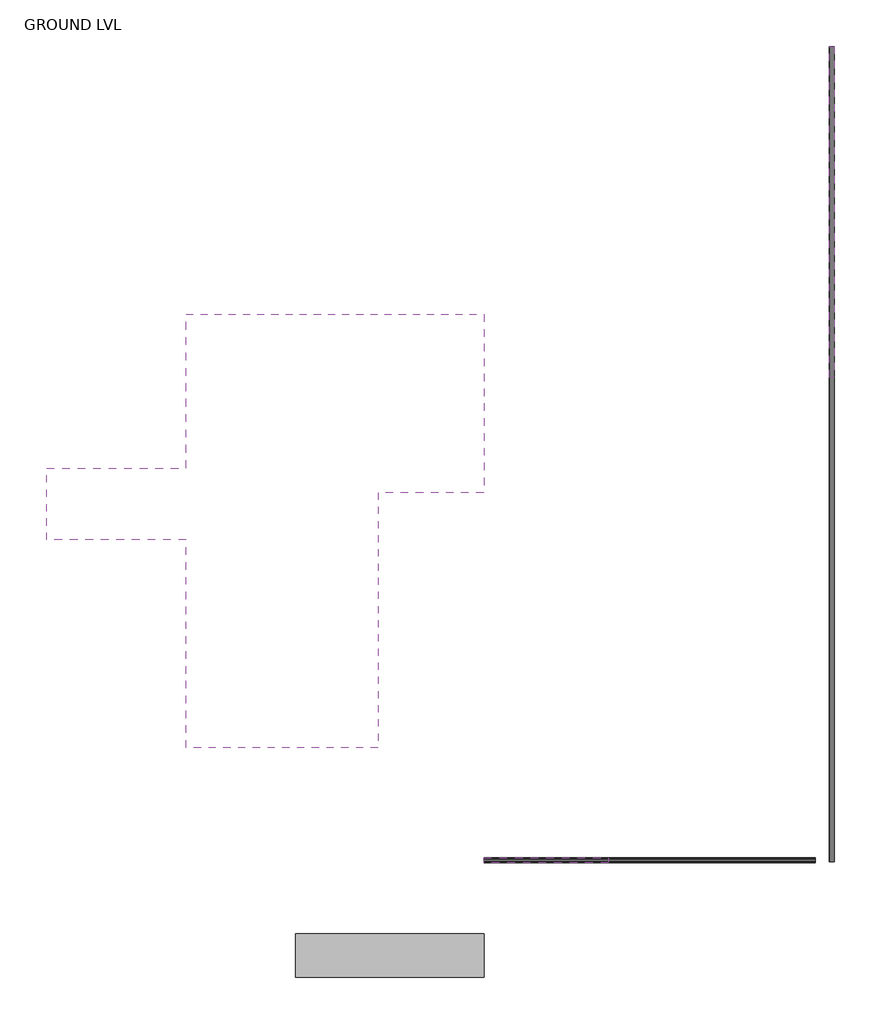
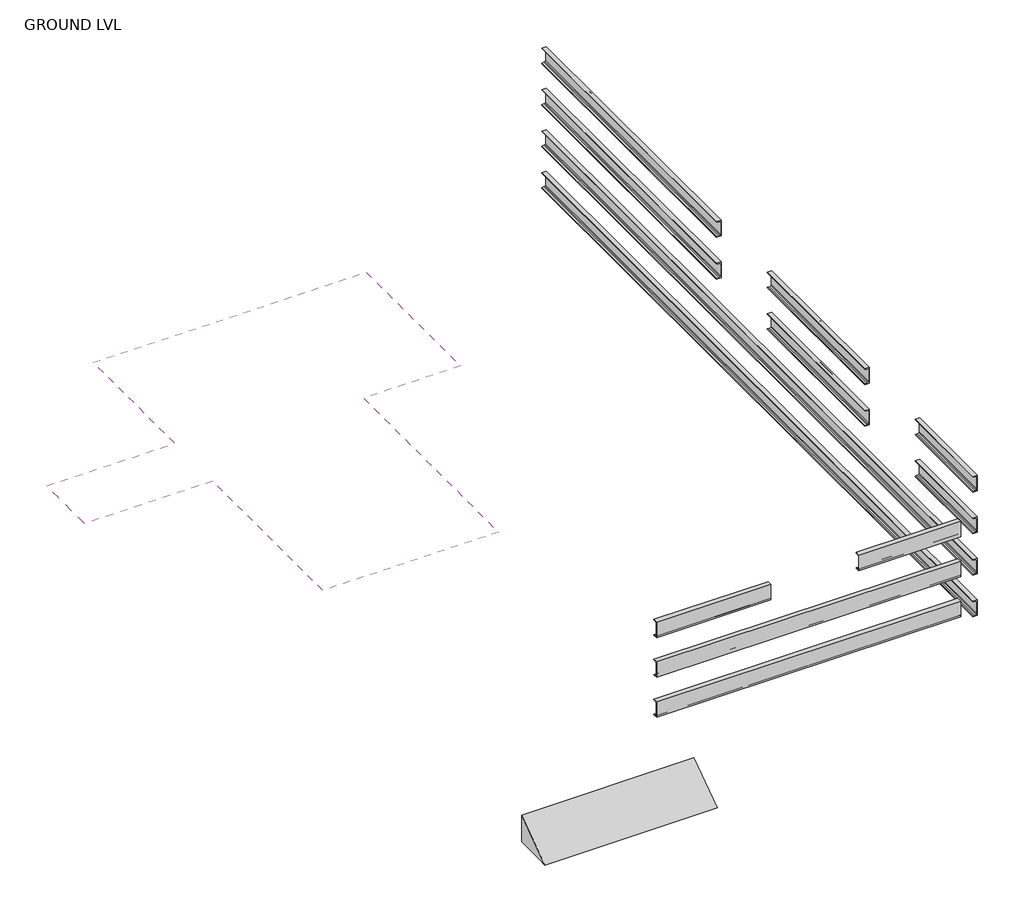
# One storey: 8 proxies, 1 covering.
"""IFC4 building model written with IfcOpenShell, lengths in millimetres."""

from ifc_helpers import new_model, si_unit, point, frame, frame_2d, origin, place, context, project, spatial, polyline, circle_curve, trimmed, segment, composite_curve, outline, extrude, transform, mapped, element, save
from components import generic_models_1_generic_models_1_f97e06e3

model = new_model("IFC4")

# Units and contexts
model_context = context("Model", 3, world=origin())
ifc_project = project(units=[si_unit("LENGTHUNIT", "METRE", prefix="MILLI")], contexts=[model_context])

# Site, building, storey
site = spatial("IfcSite", under=ifc_project)
building = spatial("IfcBuilding", under=site)
storey = spatial("IfcBuildingStorey", under=building, Name="GROUND LVL", Elevation=0.0)

# Proxies
placement = place(None, origin())
generic_models_1_generic_models_1_shape = generic_models_1_generic_models_1_f97e06e3(model_context)
element("IfcBuildingElementProxy", 1, Name="Generic Models 1 : Generic Models 1", ObjectType="Generic Models 1 : Generic Models 1", at=placement, inside=storey, context=model_context, shape_type="MappedRepresentation", body=[
    mapped(generic_models_1_generic_models_1_shape, transform((0.0, 0.0, 0.0), x_axis=(1.0, 0.0, 0.0), y_axis=(0.0, 1.0, 0.0), z_axis=(0.0, 0.0, 1.0))),
])
element("IfcBuildingElementProxy", 2, Name="Reveal", ObjectType="Reveal", at=placement, inside=storey, context=model_context, shape_type="SweptSolid", body=[
    extrude(outline(composite_curve([segment(polyline([(2425.7, -4738.2179867), (2425.7, -4801.4639867), (2424.3203242, -4801.4639867)]), True, "CONTINUOUS"), segment(trimmed(circle_curve(frame_2d((2424.3203242, -4796.2188867)), 5.2451), [point((2424.3203242, -4801.4639867))], [point((2419.1465897, -4797.0811775))], False, "CARTESIAN"), True, "CONTINUOUS"), segment(polyline([(2419.1465897, -4797.0811775), (2415.2098, -4773.4604867), (2412.00348, -4754.2226051)]), True, "CONTINUOUS"), segment(trimmed(circle_curve(frame_2d((2401.656011, -4755.9471867)), 10.4902), [point((2412.00348, -4754.2226051))], [point((2401.656011, -4745.4569867))], True, "CARTESIAN"), True, "CONTINUOUS"), segment(polyline([(2401.656011, -4745.4569867), (2221.143989, -4745.4569867)]), True, "CONTINUOUS"), segment(trimmed(circle_curve(frame_2d((2221.143989, -4755.9471867)), 10.4902), [point((2221.143989, -4745.4569867))], [point((2210.79652, -4754.2226051))], True, "CARTESIAN"), True, "CONTINUOUS"), segment(polyline([(2210.79652, -4754.2226051), (2207.5902, -4773.4604867), (2203.6534103, -4797.0811775)]), True, "CONTINUOUS"), segment(trimmed(circle_curve(frame_2d((2198.4796758, -4796.2188867)), 5.2451), [point((2203.6534103, -4797.0811775))], [point((2198.4796758, -4801.4639867))], False, "CARTESIAN"), True, "CONTINUOUS"), segment(polyline([(2198.4796758, -4801.4639867), (2197.1, -4801.4639867), (2197.1, -4738.2179867), (2425.7, -4738.2179867)]), True, "CONTINUOUS")], self_intersect=False)), frame((0.0, 4317.1500137, 0.0), z_axis=(0.0, 1.0, 0.0), x_axis=(0.0, 0.0, 1.0)), (0.0, 0.0, 1.0), 4203.7),
    extrude(outline(composite_curve([segment(polyline([(2425.7, -4738.2179867), (2425.7, -4801.4639867), (2424.3203242, -4801.4639867)]), True, "CONTINUOUS"), segment(trimmed(circle_curve(frame_2d((2424.3203242, -4796.2188867)), 5.2451), [point((2424.3203242, -4801.4639867))], [point((2419.1465897, -4797.0811775))], False, "CARTESIAN"), True, "CONTINUOUS"), segment(polyline([(2419.1465897, -4797.0811775), (2415.2098, -4773.4604867), (2412.00348, -4754.2226051)]), True, "CONTINUOUS"), segment(trimmed(circle_curve(frame_2d((2401.656011, -4755.9471867)), 10.4902), [point((2412.00348, -4754.2226051))], [point((2401.656011, -4745.4569867))], True, "CARTESIAN"), True, "CONTINUOUS"), segment(polyline([(2401.656011, -4745.4569867), (2221.143989, -4745.4569867)]), True, "CONTINUOUS"), segment(trimmed(circle_curve(frame_2d((2221.143989, -4755.9471867)), 10.4902), [point((2221.143989, -4745.4569867))], [point((2210.79652, -4754.2226051))], True, "CARTESIAN"), True, "CONTINUOUS"), segment(polyline([(2210.79652, -4754.2226051), (2207.5902, -4773.4604867), (2203.6534103, -4797.0811775)]), True, "CONTINUOUS"), segment(trimmed(circle_curve(frame_2d((2198.4796758, -4796.2188867)), 5.2451), [point((2203.6534103, -4797.0811775))], [point((2198.4796758, -4801.4639867))], False, "CARTESIAN"), True, "CONTINUOUS"), segment(polyline([(2198.4796758, -4801.4639867), (2197.1, -4801.4639867), (2197.1, -4738.2179867), (2425.7, -4738.2179867)]), True, "CONTINUOUS")], self_intersect=False)), frame((0.0, 761.1500137, 0.0), z_axis=(0.0, 1.0, 0.0), x_axis=(0.0, 0.0, 1.0)), (0.0, 0.0, 1.0), 2336.8),
    extrude(outline(composite_curve([segment(polyline([(2425.7, -4738.2179867), (2425.7, -4801.4639867), (2424.3203242, -4801.4639867)]), True, "CONTINUOUS"), segment(trimmed(circle_curve(frame_2d((2424.3203242, -4796.2188867)), 5.2451), [point((2424.3203242, -4801.4639867))], [point((2419.1465897, -4797.0811775))], False, "CARTESIAN"), True, "CONTINUOUS"), segment(polyline([(2419.1465897, -4797.0811775), (2415.2098, -4773.4604867), (2412.00348, -4754.2226051)]), True, "CONTINUOUS"), segment(trimmed(circle_curve(frame_2d((2401.656011, -4755.9471867)), 10.4902), [point((2412.00348, -4754.2226051))], [point((2401.656011, -4745.4569867))], True, "CARTESIAN"), True, "CONTINUOUS"), segment(polyline([(2401.656011, -4745.4569867), (2221.143989, -4745.4569867)]), True, "CONTINUOUS"), segment(trimmed(circle_curve(frame_2d((2221.143989, -4755.9471867)), 10.4902), [point((2221.143989, -4745.4569867))], [point((2210.79652, -4754.2226051))], True, "CARTESIAN"), True, "CONTINUOUS"), segment(polyline([(2210.79652, -4754.2226051), (2207.5902, -4773.4604867), (2203.6534103, -4797.0811775)]), True, "CONTINUOUS"), segment(trimmed(circle_curve(frame_2d((2198.4796758, -4796.2188867)), 5.2451), [point((2203.6534103, -4797.0811775))], [point((2198.4796758, -4801.4639867))], False, "CARTESIAN"), True, "CONTINUOUS"), segment(polyline([(2198.4796758, -4801.4639867), (2197.1, -4801.4639867), (2197.1, -4738.2179867), (2425.7, -4738.2179867)]), True, "CONTINUOUS")], self_intersect=False)), frame((0.0, -1842.3499863, 0.0), z_axis=(0.0, 1.0, 0.0), x_axis=(0.0, 0.0, 1.0)), (0.0, 0.0, 1.0), 1384.3),
])
element("IfcBuildingElementProxy", 3, Name="Reveal", ObjectType="Reveal", at=placement, inside=storey, context=model_context, shape_type="SweptSolid", body=[
    extrude(outline(composite_curve([segment(polyline([(-1857.2343863, 1841.5), (-1793.9883863, 1841.5), (-1793.9883863, 1840.1203242)]), True, "CONTINUOUS"), segment(trimmed(circle_curve(frame_2d((-1799.2334863, 1840.1203242)), 5.2451), [point((-1793.9883863, 1840.1203242))], [point((-1798.3711955, 1834.9465897))], False, "CARTESIAN"), True, "CONTINUOUS"), segment(polyline([(-1798.3711955, 1834.9465897), (-1821.9918863, 1831.0098), (-1841.2297679, 1827.80348)]), True, "CONTINUOUS"), segment(trimmed(circle_curve(frame_2d((-1839.5051863, 1817.456011)), 10.4902), [point((-1841.2297679, 1827.80348))], [point((-1849.9953863, 1817.456011))], True, "CARTESIAN"), True, "CONTINUOUS"), segment(polyline([(-1849.9953863, 1817.456011), (-1849.9953863, 1636.943989)]), True, "CONTINUOUS"), segment(trimmed(circle_curve(frame_2d((-1839.5051863, 1636.943989)), 10.4902), [point((-1849.9953863, 1636.943989))], [point((-1841.2297679, 1626.59652))], True, "CARTESIAN"), True, "CONTINUOUS"), segment(polyline([(-1841.2297679, 1626.59652), (-1821.9918863, 1623.3902), (-1798.3711955, 1619.4534103)]), True, "CONTINUOUS"), segment(trimmed(circle_curve(frame_2d((-1799.2334863, 1614.2796758)), 5.2451), [point((-1798.3711955, 1619.4534103))], [point((-1793.9883863, 1614.2796758))], False, "CARTESIAN"), True, "CONTINUOUS"), segment(polyline([(-1793.9883863, 1614.2796758), (-1793.9883863, 1612.9), (-1857.2343863, 1612.9), (-1857.2343863, 1841.5)]), True, "CONTINUOUS")], self_intersect=False)), frame((-6391.4023867, 0.0, 0.0), z_axis=(1.0, 0.0, 0.0), x_axis=(0.0, 1.0, 0.0)), (0.0, 0.0, 1.0), 1409.7),
    extrude(outline(composite_curve([segment(polyline([(-1857.2343863, 1841.5), (-1793.9883863, 1841.5), (-1793.9883863, 1840.1203242)]), True, "CONTINUOUS"), segment(trimmed(circle_curve(frame_2d((-1799.2334863, 1840.1203242)), 5.2451), [point((-1793.9883863, 1840.1203242))], [point((-1798.3711955, 1834.9465897))], False, "CARTESIAN"), True, "CONTINUOUS"), segment(polyline([(-1798.3711955, 1834.9465897), (-1821.9918863, 1831.0098), (-1841.2297679, 1827.80348)]), True, "CONTINUOUS"), segment(trimmed(circle_curve(frame_2d((-1839.5051863, 1817.456011)), 10.4902), [point((-1841.2297679, 1827.80348))], [point((-1849.9953863, 1817.456011))], True, "CARTESIAN"), True, "CONTINUOUS"), segment(polyline([(-1849.9953863, 1817.456011), (-1849.9953863, 1636.943989)]), True, "CONTINUOUS"), segment(trimmed(circle_curve(frame_2d((-1839.5051863, 1636.943989)), 10.4902), [point((-1849.9953863, 1636.943989))], [point((-1841.2297679, 1626.59652))], True, "CARTESIAN"), True, "CONTINUOUS"), segment(polyline([(-1841.2297679, 1626.59652), (-1821.9918863, 1623.3902), (-1798.3711955, 1619.4534103)]), True, "CONTINUOUS"), segment(trimmed(circle_curve(frame_2d((-1799.2334863, 1614.2796758)), 5.2451), [point((-1798.3711955, 1619.4534103))], [point((-1793.9883863, 1614.2796758))], False, "CARTESIAN"), True, "CONTINUOUS"), segment(polyline([(-1793.9883863, 1614.2796758), (-1793.9883863, 1612.9), (-1857.2343863, 1612.9), (-1857.2343863, 1841.5)]), True, "CONTINUOUS")], self_intersect=False)), frame((-9198.1023867, 0.0, 0.0), z_axis=(1.0, 0.0, 0.0), x_axis=(0.0, 1.0, 0.0)), (0.0, 0.0, 1.0), 1587.5),
])
element("IfcBuildingElementProxy", 4, Name="Reveal", ObjectType="Reveal", at=placement, inside=storey, context=model_context, shape_type="SweptSolid", body=[
    extrude(outline(composite_curve([segment(polyline([(-1857.2343863, 1257.3), (-1793.9883863, 1257.3), (-1793.9883863, 1255.9203242)]), True, "CONTINUOUS"), segment(trimmed(circle_curve(frame_2d((-1799.2334863, 1255.9203242)), 5.2451), [point((-1793.9883863, 1255.9203242))], [point((-1798.3711955, 1250.7465897))], False, "CARTESIAN"), True, "CONTINUOUS"), segment(polyline([(-1798.3711955, 1250.7465897), (-1821.9918863, 1246.8098), (-1841.2297679, 1243.60348)]), True, "CONTINUOUS"), segment(trimmed(circle_curve(frame_2d((-1839.5051863, 1233.256011)), 10.4902), [point((-1841.2297679, 1243.60348))], [point((-1849.9953863, 1233.256011))], True, "CARTESIAN"), True, "CONTINUOUS"), segment(polyline([(-1849.9953863, 1233.256011), (-1849.9953863, 1052.743989)]), True, "CONTINUOUS"), segment(trimmed(circle_curve(frame_2d((-1839.5051863, 1052.743989)), 10.4902), [point((-1849.9953863, 1052.743989))], [point((-1841.2297679, 1042.39652))], True, "CARTESIAN"), True, "CONTINUOUS"), segment(polyline([(-1841.2297679, 1042.39652), (-1821.9918863, 1039.1902), (-1798.3711955, 1035.2534103)]), True, "CONTINUOUS"), segment(trimmed(circle_curve(frame_2d((-1799.2334863, 1030.0796758)), 5.2451), [point((-1798.3711955, 1035.2534103))], [point((-1793.9883863, 1030.0796758))], False, "CARTESIAN"), True, "CONTINUOUS"), segment(polyline([(-1793.9883863, 1030.0796758), (-1793.9883863, 1028.7), (-1857.2343863, 1028.7), (-1857.2343863, 1257.3)]), True, "CONTINUOUS")], self_intersect=False)), frame((-9198.1023867, 0.0, 0.0), z_axis=(1.0, 0.0, 0.0), x_axis=(0.0, 1.0, 0.0)), (0.0, 0.0, 1.0), 4216.4),
])
element("IfcBuildingElementProxy", 5, Name="Reveal", ObjectType="Reveal", at=placement, inside=storey, context=model_context, shape_type="SweptSolid", body=[
    extrude(outline(composite_curve([segment(polyline([(-1857.2343863, 673.1), (-1793.9883863, 673.1), (-1793.9883863, 671.7203242)]), True, "CONTINUOUS"), segment(trimmed(circle_curve(frame_2d((-1799.2334863, 671.7203242)), 5.2451), [point((-1793.9883863, 671.7203242))], [point((-1798.3711955, 666.5465897))], False, "CARTESIAN"), True, "CONTINUOUS"), segment(polyline([(-1798.3711955, 666.5465897), (-1821.9918863, 662.6098), (-1841.2297679, 659.40348)]), True, "CONTINUOUS"), segment(trimmed(circle_curve(frame_2d((-1839.5051863, 649.056011)), 10.4902), [point((-1841.2297679, 659.40348))], [point((-1849.9953863, 649.056011))], True, "CARTESIAN"), True, "CONTINUOUS"), segment(polyline([(-1849.9953863, 649.056011), (-1849.9953863, 468.543989)]), True, "CONTINUOUS"), segment(trimmed(circle_curve(frame_2d((-1839.5051863, 468.543989)), 10.4902), [point((-1849.9953863, 468.543989))], [point((-1841.2297679, 458.19652))], True, "CARTESIAN"), True, "CONTINUOUS"), segment(polyline([(-1841.2297679, 458.19652), (-1821.9918863, 454.9902), (-1798.3711955, 451.0534103)]), True, "CONTINUOUS"), segment(trimmed(circle_curve(frame_2d((-1799.2334863, 445.8796758)), 5.2451), [point((-1798.3711955, 451.0534103))], [point((-1793.9883863, 445.8796758))], False, "CARTESIAN"), True, "CONTINUOUS"), segment(polyline([(-1793.9883863, 445.8796758), (-1793.9883863, 444.5), (-1857.2343863, 444.5), (-1857.2343863, 673.1)]), True, "CONTINUOUS")], self_intersect=False)), frame((-9198.1023867, 0.0, 0.0), z_axis=(1.0, 0.0, 0.0), x_axis=(0.0, 1.0, 0.0)), (0.0, 0.0, 1.0), 4216.4),
])
element("IfcBuildingElementProxy", 6, Name="Reveal", ObjectType="Reveal", at=placement, inside=storey, context=model_context, shape_type="SweptSolid", body=[
    extrude(outline(composite_curve([segment(polyline([(1816.1, -4738.2179867), (1816.1, -4801.4639867), (1814.7203242, -4801.4639867)]), True, "CONTINUOUS"), segment(trimmed(circle_curve(frame_2d((1814.7203242, -4796.2188867)), 5.2451), [point((1814.7203242, -4801.4639867))], [point((1809.5465897, -4797.0811775))], False, "CARTESIAN"), True, "CONTINUOUS"), segment(polyline([(1809.5465897, -4797.0811775), (1805.6098, -4773.4604867), (1802.40348, -4754.2226051)]), True, "CONTINUOUS"), segment(trimmed(circle_curve(frame_2d((1792.056011, -4755.9471867)), 10.4902), [point((1802.40348, -4754.2226051))], [point((1792.056011, -4745.4569867))], True, "CARTESIAN"), True, "CONTINUOUS"), segment(polyline([(1792.056011, -4745.4569867), (1611.543989, -4745.4569867)]), True, "CONTINUOUS"), segment(trimmed(circle_curve(frame_2d((1611.543989, -4755.9471867)), 10.4902), [point((1611.543989, -4745.4569867))], [point((1601.19652, -4754.2226051))], True, "CARTESIAN"), True, "CONTINUOUS"), segment(polyline([(1601.19652, -4754.2226051), (1597.9902, -4773.4604867), (1594.0534103, -4797.0811775)]), True, "CONTINUOUS"), segment(trimmed(circle_curve(frame_2d((1588.8796758, -4796.2188867)), 5.2451), [point((1594.0534103, -4797.0811775))], [point((1588.8796758, -4801.4639867))], False, "CARTESIAN"), True, "CONTINUOUS"), segment(polyline([(1588.8796758, -4801.4639867), (1587.5, -4801.4639867), (1587.5, -4738.2179867), (1816.1, -4738.2179867)]), True, "CONTINUOUS")], self_intersect=False)), frame((0.0, 4317.1500137, 0.0), z_axis=(0.0, 1.0, 0.0), x_axis=(0.0, 0.0, 1.0)), (0.0, 0.0, 1.0), 4203.7),
    extrude(outline(composite_curve([segment(polyline([(1816.1, -4738.2179867), (1816.1, -4801.4639867), (1814.7203242, -4801.4639867)]), True, "CONTINUOUS"), segment(trimmed(circle_curve(frame_2d((1814.7203242, -4796.2188867)), 5.2451), [point((1814.7203242, -4801.4639867))], [point((1809.5465897, -4797.0811775))], False, "CARTESIAN"), True, "CONTINUOUS"), segment(polyline([(1809.5465897, -4797.0811775), (1805.6098, -4773.4604867), (1802.40348, -4754.2226051)]), True, "CONTINUOUS"), segment(trimmed(circle_curve(frame_2d((1792.056011, -4755.9471867)), 10.4902), [point((1802.40348, -4754.2226051))], [point((1792.056011, -4745.4569867))], True, "CARTESIAN"), True, "CONTINUOUS"), segment(polyline([(1792.056011, -4745.4569867), (1611.543989, -4745.4569867)]), True, "CONTINUOUS"), segment(trimmed(circle_curve(frame_2d((1611.543989, -4755.9471867)), 10.4902), [point((1611.543989, -4745.4569867))], [point((1601.19652, -4754.2226051))], True, "CARTESIAN"), True, "CONTINUOUS"), segment(polyline([(1601.19652, -4754.2226051), (1597.9902, -4773.4604867), (1594.0534103, -4797.0811775)]), True, "CONTINUOUS"), segment(trimmed(circle_curve(frame_2d((1588.8796758, -4796.2188867)), 5.2451), [point((1594.0534103, -4797.0811775))], [point((1588.8796758, -4801.4639867))], False, "CARTESIAN"), True, "CONTINUOUS"), segment(polyline([(1588.8796758, -4801.4639867), (1587.5, -4801.4639867), (1587.5, -4738.2179867), (1816.1, -4738.2179867)]), True, "CONTINUOUS")], self_intersect=False)), frame((0.0, 761.1500137, 0.0), z_axis=(0.0, 1.0, 0.0), x_axis=(0.0, 0.0, 1.0)), (0.0, 0.0, 1.0), 2336.8),
    extrude(outline(composite_curve([segment(polyline([(1816.1, -4738.2179867), (1816.1, -4801.4639867), (1814.7203242, -4801.4639867)]), True, "CONTINUOUS"), segment(trimmed(circle_curve(frame_2d((1814.7203242, -4796.2188867)), 5.2451), [point((1814.7203242, -4801.4639867))], [point((1809.5465897, -4797.0811775))], False, "CARTESIAN"), True, "CONTINUOUS"), segment(polyline([(1809.5465897, -4797.0811775), (1805.6098, -4773.4604867), (1802.40348, -4754.2226051)]), True, "CONTINUOUS"), segment(trimmed(circle_curve(frame_2d((1792.056011, -4755.9471867)), 10.4902), [point((1802.40348, -4754.2226051))], [point((1792.056011, -4745.4569867))], True, "CARTESIAN"), True, "CONTINUOUS"), segment(polyline([(1792.056011, -4745.4569867), (1611.543989, -4745.4569867)]), True, "CONTINUOUS"), segment(trimmed(circle_curve(frame_2d((1611.543989, -4755.9471867)), 10.4902), [point((1611.543989, -4745.4569867))], [point((1601.19652, -4754.2226051))], True, "CARTESIAN"), True, "CONTINUOUS"), segment(polyline([(1601.19652, -4754.2226051), (1597.9902, -4773.4604867), (1594.0534103, -4797.0811775)]), True, "CONTINUOUS"), segment(trimmed(circle_curve(frame_2d((1588.8796758, -4796.2188867)), 5.2451), [point((1594.0534103, -4797.0811775))], [point((1588.8796758, -4801.4639867))], False, "CARTESIAN"), True, "CONTINUOUS"), segment(polyline([(1588.8796758, -4801.4639867), (1587.5, -4801.4639867), (1587.5, -4738.2179867), (1816.1, -4738.2179867)]), True, "CONTINUOUS")], self_intersect=False)), frame((0.0, -1842.3499863, 0.0), z_axis=(0.0, 1.0, 0.0), x_axis=(0.0, 0.0, 1.0)), (0.0, 0.0, 1.0), 1384.3),
])
element("IfcBuildingElementProxy", 7, Name="Reveal", ObjectType="Reveal", at=placement, inside=storey, context=model_context, shape_type="SweptSolid", body=[
    extrude(outline(composite_curve([segment(polyline([(1206.5, -4738.2179867), (1206.5, -4801.4639867), (1205.1203242, -4801.4639867)]), True, "CONTINUOUS"), segment(trimmed(circle_curve(frame_2d((1205.1203242, -4796.2188867)), 5.2451), [point((1205.1203242, -4801.4639867))], [point((1199.9465897, -4797.0811775))], False, "CARTESIAN"), True, "CONTINUOUS"), segment(polyline([(1199.9465897, -4797.0811775), (1196.0098, -4773.4604867), (1192.80348, -4754.2226051)]), True, "CONTINUOUS"), segment(trimmed(circle_curve(frame_2d((1182.456011, -4755.9471867)), 10.4902), [point((1192.80348, -4754.2226051))], [point((1182.456011, -4745.4569867))], True, "CARTESIAN"), True, "CONTINUOUS"), segment(polyline([(1182.456011, -4745.4569867), (1001.943989, -4745.4569867)]), True, "CONTINUOUS"), segment(trimmed(circle_curve(frame_2d((1001.943989, -4755.9471867)), 10.4902), [point((1001.943989, -4745.4569867))], [point((991.59652, -4754.2226051))], True, "CARTESIAN"), True, "CONTINUOUS"), segment(polyline([(991.59652, -4754.2226051), (988.3902, -4773.4604867), (984.4534103, -4797.0811775)]), True, "CONTINUOUS"), segment(trimmed(circle_curve(frame_2d((979.2796758, -4796.2188867)), 5.2451), [point((984.4534103, -4797.0811775))], [point((979.2796758, -4801.4639867))], False, "CARTESIAN"), True, "CONTINUOUS"), segment(polyline([(979.2796758, -4801.4639867), (977.9, -4801.4639867), (977.9, -4738.2179867), (1206.5, -4738.2179867)]), True, "CONTINUOUS")], self_intersect=False)), frame((0.0, -1842.3499863, 0.0), z_axis=(0.0, 1.0, 0.0), x_axis=(0.0, 0.0, 1.0)), (0.0, 0.0, 1.0), 10363.2),
])
element("IfcBuildingElementProxy", 8, Name="Reveal", ObjectType="Reveal", at=placement, inside=storey, context=model_context, shape_type="SweptSolid", body=[
    extrude(outline(composite_curve([segment(polyline([(596.9, -4738.2179867), (596.9, -4801.4639867), (595.5203242, -4801.4639867)]), True, "CONTINUOUS"), segment(trimmed(circle_curve(frame_2d((595.5203242, -4796.2188867)), 5.2451), [point((595.5203242, -4801.4639867))], [point((590.3465897, -4797.0811775))], False, "CARTESIAN"), True, "CONTINUOUS"), segment(polyline([(590.3465897, -4797.0811775), (586.4098, -4773.4604867), (583.20348, -4754.2226051)]), True, "CONTINUOUS"), segment(trimmed(circle_curve(frame_2d((572.856011, -4755.9471867)), 10.4902), [point((583.20348, -4754.2226051))], [point((572.856011, -4745.4569867))], True, "CARTESIAN"), True, "CONTINUOUS"), segment(polyline([(572.856011, -4745.4569867), (392.343989, -4745.4569867)]), True, "CONTINUOUS"), segment(trimmed(circle_curve(frame_2d((392.343989, -4755.9471867)), 10.4902), [point((392.343989, -4745.4569867))], [point((381.99652, -4754.2226051))], True, "CARTESIAN"), True, "CONTINUOUS"), segment(polyline([(381.99652, -4754.2226051), (378.7902, -4773.4604867), (374.8534103, -4797.0811775)]), True, "CONTINUOUS"), segment(trimmed(circle_curve(frame_2d((369.6796758, -4796.2188867)), 5.2451), [point((374.8534103, -4797.0811775))], [point((369.6796758, -4801.4639867))], False, "CARTESIAN"), True, "CONTINUOUS"), segment(polyline([(369.6796758, -4801.4639867), (368.3, -4801.4639867), (368.3, -4738.2179867), (596.9, -4738.2179867)]), True, "CONTINUOUS")], self_intersect=False)), frame((0.0, -1842.3499863, 0.0), z_axis=(0.0, 1.0, 0.0), x_axis=(0.0, 0.0, 1.0)), (0.0, 0.0, 1.0), 10363.2),
])

# Covering
element("IfcCovering", 9, ObjectType="GWB on Mtl. Stud 2", at=placement, inside=storey, context=model_context, shape_type="SweptSolid", body=[
    extrude(outline(polyline([(-12982.7023867, 2246.6265627), (-14760.7023867, 2246.6265627), (-14760.7023867, 3161.4500137), (-12982.7023867, 3161.4500137), (-12982.7023867, 5117.2500137), (-9198.1023867, 5117.2500137), (-9198.1023867, 2848.1833471), (-10544.3023867, 2848.1833471), (-10544.3023867, -394.5499863), (-12982.7023867, -394.5499863), (-12982.7023867, 2246.6265627)])), frame((0.0, 0.0, 2743.2), z_axis=(0.0, 0.0, 1.0), x_axis=(1.0, 0.0, 0.0)), (0.0, 0.0, 1.0), 107.95),
])

save(model, "model.ifc")

# Revit data of these elements
# Type "GWB on Mtl. Stud 2"
#   Assembly Code = "C3030220"
#   built-in parameter 1002203 = 1 (stored number, unit not read)
#   built-in parameter 1002202 = 1 (stored number, unit not read)
#   Layers, outside or top first: 0' - 3 5/8" "Metal Stud Layer" (function 1); 0' - 0 5/8" "Tile, Porcelain, 4in" (function 5)
# Element 1 (IfcBuildingElementProxy, "Generic Models 1 : Generic Models 1")
#   Phase Created = New Construction
#   Materials on its faces: "Tile, Porcelain, 4in"
# Element 9 (IfcCovering, "GWB on Mtl. Stud 2")
#   Height Offset From Level = 9' - 0"
#   Phase Created = New Construction
#   Materials on its faces: "Tile, Porcelain, 4in", "Metal Stud Layer"
# Materials
#   "Metal Stud Layer": class "Metal", colour RGB 199 199 199, transparency 0, Description = "Light gauge steel framing, thermal air layer", Cost = 0
#   "Tile, Porcelain, 4in": class "Generic", colour RGB 89 87 158, transparency 0, Description = "Porcelain tile, 4\", white", Cost = 0
